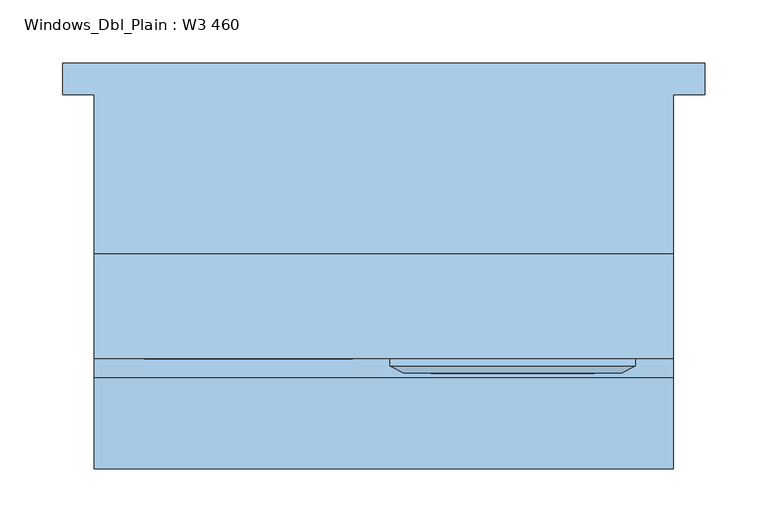
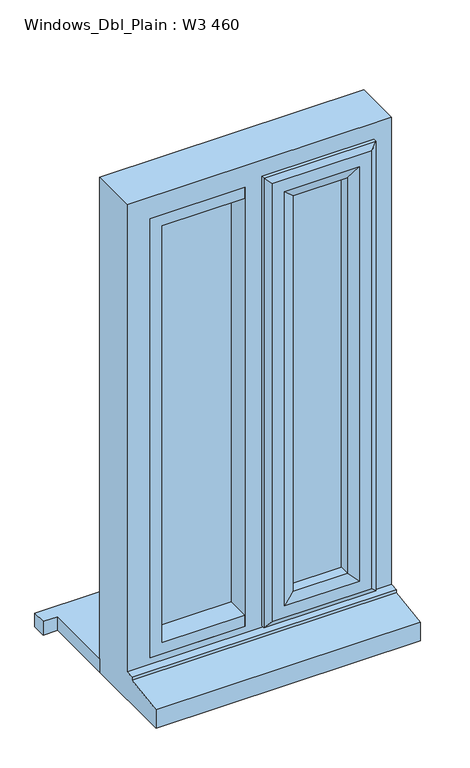
"""IFC4 building model written with IfcOpenShell, lengths in millimetres: window geometry, Windows_Dbl_Plain : W3 460."""

from ifc_helpers import new_model, si_unit, frame, origin, place, context, project, spatial, polyline, outline, extrude, faceted_brep, source, transform, mapped, element, save


def windows_dbl_plain_w3_460_956a2ca0(model_context):
    return source(origin(), model_context, "Body", "SolidModel", [
        extrude(outline(polyline([(-540.0, 146.5434322), (-30.0, 146.5434322), (-30.0, 121.5434322), (-55.0, 121.5434322), (-55.0, -5.4565678), (-515.0, -5.4565678), (-515.0, 121.5434322), (-540.0, 121.5434322), (-540.0, 146.5434322)])), frame((0.0, 0.0, 1200.0), z_axis=(0.0, 0.0, 1.0), x_axis=(1.0, 0.0, 0.0)), (0.0, 0.0, 1.0), 25.0),
        faceted_brep([(-280.0, -88.4565678, 2080.0), (-280.0, -88.4565678, 1253.0), (-280.0, -94.2300705, 1253.0), (-280.0, -94.2300705, 2080.0), (-270.0, -23.4565678, 2070.0), (-270.0, -23.4565678, 1263.0), (-270.0, -88.4565678, 1263.0), (-270.0, -88.4565678, 2070.0), (-230.0, -37.9494677, 2030.0), (-230.0, -37.9494677, 1303.0), (-240.1480377, -23.4565678, 1292.8519623), (-240.1480377, -23.4565678, 2040.1480377), (-230.0, -52.4565678, 2030.0), (-230.0, -52.4565678, 1303.0), (-240.0, -76.4565678, 2040.0), (-240.0, -76.4565678, 1293.0), (-240.0, -52.4565678, 1293.0), (-240.0, -52.4565678, 2040.0), (-230.0, -94.2300705, 2030.0), (-230.0, -94.2300705, 1303.0), (-230.0, -76.4565678, 1303.0), (-230.0, -76.4565678, 2030.0), (-247.4457548, -100.0035732, 2047.4457548), (-247.4457548, -100.0035732, 1285.5542452), (-269.2153903, -100.0035732, 1263.7846097), (-269.2153903, -100.0035732, 2069.2153903), (-85.0, -88.4565678, 1253.0), (-85.0, -94.2300705, 1253.0), (-95.0, -23.4565678, 1263.0), (-95.0, -88.4565678, 1263.0), (-135.0, -37.9494677, 1303.0), (-124.8519623, -23.4565678, 1292.8519623), (-135.0, -52.4565678, 1303.0), (-125.0, -76.4565678, 1293.0), (-125.0, -52.4565678, 1293.0), (-135.0, -94.2300705, 1303.0), (-135.0, -76.4565678, 1303.0), (-117.5542452, -100.0035732, 1285.5542452), (-95.7846097, -100.0035732, 1263.7846097), (-85.0, -88.4565678, 2080.0), (-85.0, -94.2300705, 2080.0), (-95.0, -23.4565678, 2070.0), (-95.0, -88.4565678, 2070.0), (-135.0, -37.9494677, 2030.0), (-124.8519623, -23.4565678, 2040.1480377), (-135.0, -52.4565678, 2030.0), (-125.0, -76.4565678, 2040.0), (-125.0, -52.4565678, 2040.0), (-135.0, -94.2300705, 2030.0), (-135.0, -76.4565678, 2030.0), (-117.5542452, -100.0035732, 2047.4457548), (-95.7846097, -100.0035732, 2069.2153903)], [[[0, 1, 2, 3]], [[4, 5, 6, 7]], [[8, 9, 10, 11]], [[12, 13, 9, 8]], [[14, 15, 16, 17]], [[18, 19, 20, 21]], [[22, 23, 19, 18]], [[3, 2, 24, 25]], [[1, 26, 27, 2]], [[5, 28, 29, 6]], [[9, 30, 31, 10]], [[13, 32, 30, 9]], [[15, 33, 34, 16]], [[19, 35, 36, 20]], [[23, 37, 35, 19]], [[2, 27, 38, 24]], [[26, 39, 40, 27]], [[28, 41, 42, 29]], [[30, 43, 44, 31]], [[32, 45, 43, 30]], [[33, 46, 47, 34]], [[35, 48, 49, 36]], [[37, 50, 48, 35]], [[27, 40, 51, 38]], [[39, 0, 3, 40]], [[1, 0, 39, 26], [7, 6, 29, 42]], [[41, 4, 7, 42]], [[5, 4, 41, 28], [11, 10, 31, 44]], [[43, 8, 11, 44]], [[45, 12, 8, 43]], [[17, 16, 34, 47], [13, 12, 45, 32]], [[46, 14, 17, 47]], [[15, 14, 46, 33], [21, 20, 36, 49]], [[48, 18, 21, 49]], [[50, 22, 18, 48]], [[25, 24, 38, 51], [23, 22, 50, 37]], [[40, 3, 25, 51]]]),
        extrude(outline(polyline([(2070.0, -310.0), (2070.0, -475.0), (1263.0, -475.0), (1263.0, -310.0), (1283.0, -310.0), (1283.0, -455.0), (2050.0, -455.0), (2050.0, -310.0), (2070.0, -310.0)])), frame((0.0, -88.4565678, 0.0), z_axis=(0.0, 1.0, 0.0), x_axis=(0.0, 0.0, 1.0)), (0.0, 0.0, 1.0), 41.0),
        faceted_brep([(-55.0, -5.4565678, 2110.0), (-55.0, -5.4565678, 1200.0), (-515.0, -5.4565678, 1200.0), (-515.0, -5.4565678, 2110.0), (-115.0, -5.4565678, 2050.0), (-252.0, -5.4565678, 2050.0), (-252.0, -5.4565678, 1275.0), (-115.0, -5.4565678, 1275.0), (-310.0, -5.4565678, 2050.0), (-455.0, -5.4565678, 2050.0), (-455.0, -5.4565678, 1275.0), (-310.0, -5.4565678, 1275.0), (-515.0, -175.9565678, 1200.0), (-515.0, -175.9565678, 1233.8088847), (-515.0, -103.4565678, 1244.7449676), (-515.0, -103.4565678, 1249.68767), (-515.0, -88.4565678, 1251.0), (-515.0, -88.4565678, 2110.0), (-55.0, -88.4565678, 1251.0), (-55.0, -88.4565678, 2110.0), (-475.0, -88.4565678, 2070.0), (-310.0, -88.4565678, 2070.0), (-310.0, -88.4565678, 1263.0), (-475.0, -88.4565678, 1263.0), (-270.0, -88.4565678, 2070.0), (-95.0, -88.4565678, 2070.0), (-95.0, -88.4565678, 1263.0), (-270.0, -88.4565678, 1263.0), (-475.0, -23.4565678, 1263.0), (-475.0, -23.4565678, 2070.0), (-300.0, -23.4565678, 1263.0), (-300.0, -23.4565678, 2070.0), (-310.0, -23.4565678, 2050.0), (-310.0, -23.4565678, 1275.0), (-455.0, -23.4565678, 1275.0), (-455.0, -23.4565678, 2050.0), (-270.0, -23.4565678, 2070.0), (-270.0, -23.4565678, 1263.0), (-95.0, -23.4565678, 1263.0), (-95.0, -23.4565678, 2070.0), (-115.0, -23.4565678, 2050.0), (-115.0, -23.4565678, 1275.0), (-252.0, -23.4565678, 1275.0), (-252.0, -23.4565678, 2050.0), (-300.0, -47.4565678, 2070.0), (-310.0, -47.4565678, 2070.0), (-55.0, -103.4565678, 1249.68767), (-55.0, -103.4565678, 1244.7449676), (-55.0, -175.9565678, 1233.8088847), (-55.0, -175.9565678, 1200.0), (-300.0, -47.4565678, 1263.0), (-310.0, -47.4565678, 1263.0)], [[[0, 1, 2, 3], [4, 5, 6, 7], [8, 9, 10, 11]], [[2, 12, 13, 14, 15, 16, 17, 3]], [[16, 18, 19, 17], [20, 21, 22, 23], [24, 25, 26, 27]], [[23, 28, 29, 20]], [[29, 28, 30, 31], [32, 33, 34, 35]], [[36, 37, 38, 39], [40, 41, 42, 43]], [[35, 34, 10, 9]], [[3, 17, 19, 0]], [[25, 24, 36, 39]], [[29, 31, 44, 45, 21, 20]], [[9, 8, 32, 35]], [[40, 43, 5, 4]], [[18, 46, 47, 48, 49, 1, 0, 19]], [[25, 39, 38, 26]], [[4, 7, 41, 40]], [[44, 31, 30, 50]], [[50, 51, 45, 44]], [[51, 22, 21, 45]], [[27, 37, 36, 24]], [[43, 42, 6, 5]], [[8, 11, 33, 32]], [[49, 12, 2, 1]], [[48, 13, 12, 49]], [[47, 14, 13, 48]], [[46, 15, 14, 47]], [[18, 16, 15, 46]], [[26, 38, 37, 27]], [[22, 51, 50, 30, 28, 23]], [[6, 42, 41, 7]], [[33, 11, 10, 34]]]),
        extrude(outline(polyline([(-475.0, -47.4565678), (-475.0, -23.4565678), (-300.0, -23.4565678), (-300.0, -47.4565678), (-475.0, -47.4565678)])), frame((0.0, 0.0, 1263.0), z_axis=(0.0, 0.0, 1.0), x_axis=(1.0, 0.0, 0.0)), (0.0, 0.0, 1.0), 807.0),
        extrude(outline(polyline([(-125.0, -52.4565678), (-125.0, -76.4565678), (-240.0, -76.4565678), (-240.0, -52.4565678), (-125.0, -52.4565678)])), frame((0.0, 0.0, 1293.0), z_axis=(0.0, 0.0, 1.0), x_axis=(1.0, 0.0, 0.0)), (0.0, 0.0, 1.0), 747.0),
    ])


if __name__ == "__main__":
    model = new_model("IFC4")
    model_context = context("Model", 3, world=origin())
    ifc_project = project(units=[si_unit("LENGTHUNIT", "METRE", prefix="MILLI")], contexts=[model_context])
    site = spatial("IfcSite", under=ifc_project)
    building = spatial("IfcBuilding", under=site)
    placement = place(None, origin())
    windows_dbl_plain_w3_460_shape = windows_dbl_plain_w3_460_956a2ca0(model_context)
    element("IfcWindow", 1, ObjectType="Windows_Dbl_Plain : W3 460", at=placement, inside=building, context=model_context, shape_type="MappedRepresentation", body=[
        mapped(windows_dbl_plain_w3_460_shape, transform((0.0, 0.0, 0.0), x_axis=(1.0, 0.0, 0.0), y_axis=(0.0, 1.0, 0.0), z_axis=(0.0, 0.0, 1.0))),
    ])
    save(model, "model.ifc")

# Revit data of these elements
# Type "Windows_Dbl_Plain : W3 460"
#   Type Mark = "64"
#   Operation = "DoublePanelVertical"
#   Construction Type Id = "GSP4R"
#   Manufacturer = "Revit"
#   Keynote = "L10"
#   Analytic Construction = "1/8 in Pilkington single glazing"
#   Wrap Layers (Ext) from Ext = 102.5 mm
#   Wrap Layers (Int) from Ext = 177.5 mm
#   Window Board Projection = 25 mm
#   Window Board Extension = 25 mm
#   Visual Light Transmittance = 0.9
#   Solar Heat Gain Coefficient = 0.78
#   Rough Width = 460 mm
#   Rough Height = 910 mm
#   Height = 910 mm
#   Width = 460 mm
#   Heat Transfer Coefficient (U) = 3.6886 W/(m²·K)
#   Glazing Thickness = 24 mm
#   FrameOffset - External = 50 mm
#   Frame Depth = 65 mm
#   Default Head Height = 2110 mm
#   Cill Depth = 87.5 mm
#   Cavity Closer Width = 50 mm
#   Cavity Closer Offset from Ext = 102.5 mm
#   Cavity Closer Depth = 85 mm
#   Vis - Cavity Closers = yes
#   Define Thermal Properties by = 1
#   Material Trim = Window Frame
#   Material Glass = Glass
#   Material Frame = Window Frame
#   Wall Closure = (empty or 0)
# Element 1 (IfcWindow, "Windows_Dbl_Plain : W3 460")
#   Materials on its faces: "Window Frame", "Glass"
# Materials
#   "Window Frame": colour RGB 249 249 249, transparency 0, Keynote = "L10", Cost = 0
#   "Glass": class "Glass", colour RGB 0 128 192, transparency 0.9, Description = "Soda Lime Glass", Cost = 0
